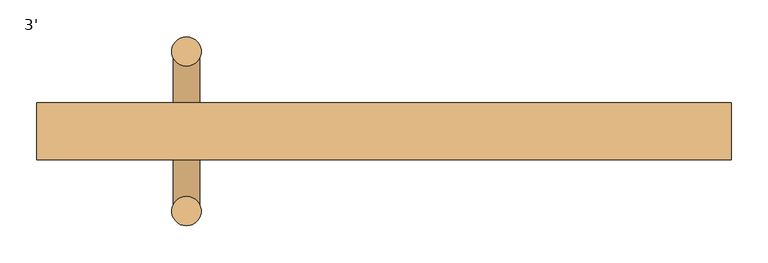
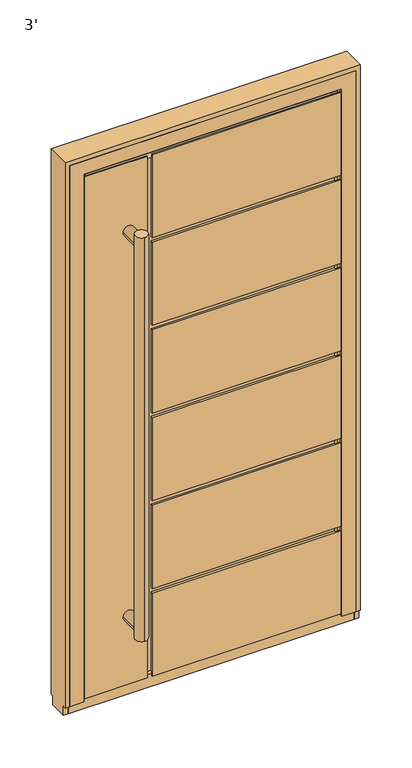
"""IFC4 building model written with IfcOpenShell, lengths in millimetres: door geometry, 3'."""

from ifc_helpers import new_model, si_unit, point, frame, frame_2d, origin, place, context, project, spatial, circle_curve, trimmed, segment, composite_curve, outline, extrude, faceted_brep, source, transform, mapped, element, save


def door_3_3562bf2b(model_context):
    return source(origin(), model_context, "Body", "SolidModel", [
        extrude(outline(composite_curve([segment(trimmed(circle_curve(frame_2d((-268.65, 52.7003001)), 20.0), [point((-268.65, 32.7003001))], [point((-268.65, 72.7003001))], False, "CARTESIAN"), True, "CONTINUOUS"), segment(trimmed(circle_curve(frame_2d((-268.65, 52.7003001)), 20.0), [point((-268.65, 72.7003001))], [point((-268.65, 32.7003001))], False, "CARTESIAN"), True, "CONTINUOUS")], self_intersect=False)), frame((0.0, 0.0, 210.0000003), z_axis=(0.0, 0.0, 1.0), x_axis=(1.0, 0.0, 0.0)), (0.0, 0.0, 1.0), 1363.8),
        extrude(outline(composite_curve([segment(trimmed(circle_curve(frame_2d((-268.65, -164.3003001)), 20.0), [point((-268.65, -184.3003001))], [point((-268.65, -144.3003001))], False, "CARTESIAN"), True, "CONTINUOUS"), segment(trimmed(circle_curve(frame_2d((-268.65, -164.3003001)), 20.0), [point((-268.65, -144.3003001))], [point((-268.65, -184.3003001))], False, "CARTESIAN"), True, "CONTINUOUS")], self_intersect=False)), frame((0.0, 0.0, 210.0000003), z_axis=(0.0, 0.0, 1.0), x_axis=(1.0, 0.0, 0.0)), (0.0, 0.0, 1.0), 1363.8),
        extrude(outline(composite_curve([segment(trimmed(circle_curve(frame_2d((241.9000003, -268.65)), 18.0), [point((241.9000003, -286.65))], [point((241.9000003, -250.65))], False, "CARTESIAN"), True, "CONTINUOUS"), segment(trimmed(circle_curve(frame_2d((241.9000003, -268.65)), 18.0), [point((241.9000003, -250.65))], [point((241.9000003, -286.65))], False, "CARTESIAN"), True, "CONTINUOUS")], self_intersect=False)), frame((0.0, -164.3, 0.0), z_axis=(0.0, 1.0, 0.0), x_axis=(0.0, 0.0, 1.0)), (0.0, 0.0, 1.0), 217.0),
        extrude(outline(composite_curve([segment(trimmed(circle_curve(frame_2d((1541.9000003, -268.65)), 18.0), [point((1541.9000003, -286.65))], [point((1541.9000003, -250.65))], False, "CARTESIAN"), True, "CONTINUOUS"), segment(trimmed(circle_curve(frame_2d((1541.9000003, -268.65)), 18.0), [point((1541.9000003, -250.65))], [point((1541.9000003, -286.65))], False, "CARTESIAN"), True, "CONTINUOUS")], self_intersect=False)), frame((0.0, -164.3, 0.0), z_axis=(0.0, 1.0, 0.0), x_axis=(0.0, 0.0, 1.0)), (0.0, 0.0, 1.0), 217.0),
        faceted_brep([(-193.65, -24.3, 306.466667), (383.65, -24.3, 306.466667), (383.65, -24.3, 291.466667), (-193.65, -24.3, 291.466667), (-193.65, -24.3, 35.0), (-208.65, -24.3, 35.0), (-208.65, -24.3, 1748.8000003), (-193.65, -24.3, 1748.8000003), (-193.65, -24.3, 1492.3333337), (383.65, -24.3, 1492.3333337), (383.65, -24.3, 1477.3333337), (-193.65, -24.3, 1477.3333337), (-193.65, -24.3, 1195.866667), (383.65, -24.3, 1195.866667), (383.65, -24.3, 1180.866667), (-193.65, -24.3, 1180.866667), (-193.65, -24.3, 899.4000004), (383.65, -24.3, 899.4000004), (383.65, -24.3, 884.4000004), (-193.65, -24.3, 884.4000004), (-193.65, -24.3, 602.9333337), (383.65, -24.3, 602.9333337), (383.65, -24.3, 587.9333337), (-193.65, -24.3, 587.9333337), (-193.65, -17.3, 587.9333337), (-193.65, -17.3, 306.466667), (383.65, -17.3, 587.9333337), (383.65, -26.3002302, 1748.8000003), (383.65, -26.3002302, 35.0), (383.65, -19.2979528, 35.0), (383.65, -19.2979528, 24.0), (383.65, -17.3, 24.0), (383.65, -17.3, 291.466667), (383.65, -17.3, 306.466667), (383.65, -17.3, 602.9333337), (383.65, -17.3, 884.4000004), (383.65, -17.3, 899.4000004), (383.65, -17.3, 1180.866667), (383.65, -17.3, 1195.866667), (383.65, -17.3, 1477.3333337), (383.65, -17.3, 1492.3333337), (383.65, -17.3, 1748.8000003), (-193.65, -17.3, 602.9333337), (-193.65, -17.3, 884.4000004), (-193.65, -17.3, 899.4000004), (-193.65, -17.3, 1180.866667), (-208.65, -19.2979528, 35.0), (-208.65, -19.2979528, 24.0), (-208.65, -17.3, 24.0), (-208.65, -17.3, 1748.8000003), (-383.65, -26.3002302, 35.0), (-383.65, -19.2979528, 35.0), (-193.65, -19.2979528, 35.0), (-193.65, -17.3, 291.466667), (-193.65, -17.3, 24.0), (-193.65, -19.2979528, 24.0), (-383.65, -19.2979528, 24.0), (-383.65, -17.3, 24.0), (-383.65, -17.3, 1748.8000003), (-193.65, -17.3, 1195.866667), (-193.65, -17.3, 1477.3333337), (-193.65, -17.3, 1492.3333337), (-193.65, -17.3, 1748.8000003), (408.65, -94.3, 10.0000003), (-193.65, -94.3, 10.0000003), (-193.65, -91.3, 10.0000003), (408.65, -91.3, 10.0000003), (-408.65, -91.3, 10.0000003), (-208.65, -91.3, 10.0000003), (-208.65, -94.3, 10.0000003), (-408.65, -94.3, 10.0000003), (408.65, -94.3, 306.466667), (408.65, -91.3, 306.466667), (408.65, -91.3, 587.9333337), (408.65, -94.3, 587.9333337), (408.65, -94.3, 899.4000004), (408.65, -91.3, 899.4000004), (408.65, -91.3, 1180.866667), (408.65, -94.3, 1180.866667), (408.65, -94.3, 602.9333337), (408.65, -91.3, 602.9333337), (408.65, -91.3, 884.4000004), (408.65, -94.3, 884.4000004), (408.65, -94.3, 1195.866667), (408.65, -91.3, 1195.866667), (408.65, -91.3, 1477.3333337), (408.65, -94.3, 1477.3333337), (408.65, -94.3, 1773.8000003), (408.65, -94.3, 1492.3333337), (408.65, -91.3, 1492.3333337), (408.65, -91.3, 1773.8000003), (408.65, -91.3, 291.466667), (408.65, -94.3, 291.466667), (-193.65, -91.3, 25.5), (393.15, -91.3, 25.5), (393.15, -91.3, 291.466667), (393.15, -91.3, 306.466667), (393.15, -91.3, 587.9333337), (393.15, -91.3, 899.4000004), (393.15, -91.3, 1180.866667), (393.15, -91.3, 602.9333337), (393.15, -91.3, 884.4000004), (-393.15, -91.3, 25.5), (-208.65, -91.3, 25.5), (-408.65, -91.3, 1773.8000003), (-208.65, -91.3, 1773.8000003), (-208.65, -91.3, 1758.3000003), (-393.15, -91.3, 1758.3000003), (393.15, -91.3, 1195.866667), (393.15, -91.3, 1477.3333337), (393.15, -91.3, 1492.3333337), (393.15, -91.3, 1758.3000003), (-193.65, -91.3, 1758.3000003), (-193.65, -91.3, 1773.8000003), (-193.65, -87.3, 291.466667), (-193.65, -87.3, 25.5), (-193.65, -94.3, 291.466667), (-208.65, -94.3, 1773.8000003), (-408.65, -94.3, 1773.8000003), (-193.65, -94.3, 587.9333337), (-193.65, -94.3, 306.466667), (-193.65, -94.3, 1180.866667), (-193.65, -94.3, 899.4000004), (-193.65, -94.3, 884.4000004), (-193.65, -94.3, 602.9333337), (-193.65, -94.3, 1477.3333337), (-193.65, -94.3, 1195.866667), (-193.65, -94.3, 1773.8000003), (-193.65, -94.3, 1492.3333337), (-208.65, -87.3, 1758.3000003), (-208.65, -87.3, 25.5), (-383.65, -26.3002302, 1748.8000003), (393.15, -26.3002302, 1758.3000003), (393.15, -26.3002302, 25.5), (-393.15, -26.3002302, 25.5), (-393.15, -26.3002302, 1758.3000003), (393.15, -87.3, 1492.3333337), (393.15, -87.3, 1477.3333337), (393.15, -87.3, 1195.866667), (393.15, -87.3, 1180.866667), (393.15, -87.3, 899.4000004), (393.15, -87.3, 884.4000004), (393.15, -87.3, 602.9333337), (393.15, -87.3, 587.9333337), (393.15, -87.3, 306.466667), (393.15, -87.3, 291.466667), (-193.65, -87.3, 1477.3333337), (-193.65, -87.3, 1492.3333337), (-193.65, -87.3, 1758.3000003), (-193.65, -87.3, 306.466667), (-193.65, -87.3, 587.9333337), (-193.65, -87.3, 602.9333337), (-193.65, -87.3, 884.4000004), (-193.65, -87.3, 899.4000004), (-193.65, -87.3, 1180.866667), (-193.65, -87.3, 1195.866667)], [[[0, 1, 2, 3, 4, 5, 6, 7, 8, 9, 10, 11, 12, 13, 14, 15, 16, 17, 18, 19, 20, 21, 22, 23]], [[23, 24, 25, 0]], [[23, 22, 26, 24]], [[27, 28, 29, 30, 31, 32, 2, 1, 33, 26, 22, 21, 34, 35, 18, 17, 36, 37, 14, 13, 38, 39, 10, 9, 40, 41]], [[42, 34, 21, 20]], [[19, 43, 42, 20]], [[19, 18, 35, 43]], [[44, 36, 17, 16]], [[15, 45, 44, 16]], [[5, 46, 47, 48, 49, 6]], [[28, 50, 51, 46, 5, 4, 52, 29]], [[53, 54, 55, 52, 4, 3]], [[3, 2, 32, 53]], [[25, 33, 1, 0]], [[29, 52, 55, 30]], [[56, 47, 46, 51]], [[30, 55, 54, 31]], [[57, 48, 47, 56]], [[36, 44, 45, 37]], [[34, 42, 43, 35]], [[33, 25, 24, 26]], [[54, 53, 32, 31]], [[58, 49, 48, 57]], [[38, 59, 60, 39]], [[41, 40, 61, 62]], [[63, 64, 65, 66]], [[67, 68, 69, 70]], [[71, 72, 73, 74]], [[75, 76, 77, 78]], [[79, 80, 81, 82]], [[83, 84, 85, 86]], [[87, 88, 89, 90]], [[66, 91, 92, 63]], [[65, 93, 94, 95, 91, 66]], [[72, 96, 97, 73]], [[76, 98, 99, 77]], [[80, 100, 101, 81]], [[102, 103, 68, 67, 104, 105, 106, 107]], [[84, 108, 109, 85]], [[90, 89, 110, 111, 112, 113]], [[114, 115, 93, 65, 64, 116]], [[70, 69, 117, 118]], [[63, 92, 116, 64]], [[74, 119, 120, 71]], [[78, 121, 122, 75]], [[82, 123, 124, 79]], [[86, 125, 126, 83]], [[87, 127, 128, 88]], [[70, 118, 104, 67]], [[129, 106, 105, 117, 69, 68, 103, 130]], [[58, 57, 56, 51, 50, 131]], [[132, 133, 134, 135], [131, 50, 28, 27]], [[111, 110, 136, 137, 109, 108, 138, 139, 99, 98, 140, 141, 101, 100, 142, 143, 97, 96, 144, 145, 95, 94, 133, 132]], [[94, 93, 115, 130, 103, 102, 134, 133]], [[135, 134, 102, 107]], [[146, 137, 136, 147, 148, 129, 130, 115, 114, 145, 144, 149, 150, 143, 142, 151, 152, 141, 140, 153, 154, 139, 138, 155]], [[153, 122, 121, 154]], [[153, 140, 98, 76, 75, 122]], [[123, 82, 81, 101, 141, 152]], [[151, 124, 123, 152]], [[151, 142, 100, 80, 79, 124]], [[119, 74, 73, 97, 143, 150]], [[149, 120, 119, 150]], [[149, 144, 96, 72, 71, 120]], [[116, 92, 91, 95, 145, 114]], [[15, 14, 37, 45]], [[59, 38, 13, 12]], [[11, 60, 59, 12]], [[11, 10, 39, 60]], [[61, 40, 9, 8]], [[8, 7, 62, 61]], [[125, 86, 85, 109, 137, 146]], [[128, 127, 113, 112, 148, 147]], [[121, 78, 77, 99, 139, 154]], [[155, 138, 108, 84, 83, 126]], [[155, 126, 125, 146]], [[147, 136, 110, 89, 88, 128]], [[90, 113, 127, 87]], [[118, 117, 105, 104]], [[132, 135, 107, 106, 129, 148, 112, 111]], [[27, 41, 62, 7, 6, 49, 58, 131]]]),
        faceted_brep([(-457.2, -94.3, 0.0), (-457.2, -85.2997571, 0.0), (-412.7, -85.2997571, 0.0), (-412.7, -94.3, 0.0), (-403.2, -21.8000042, 0.0), (-403.2, -26.3, 0.0), (-457.2, -26.3, 0.0), (-457.2, -17.3, 0.0), (-387.7, -17.3, 0.0), (-387.7, -21.8000042, 0.0), (457.2, -17.3, 0.0), (457.2, -26.3, 0.0), (403.2, -26.3, 0.0), (403.2, -21.8000042, 0.0), (387.7, -21.8000042, 0.0), (387.7, -17.3, 0.0), (412.7, -85.2997571, 0.0), (457.2, -85.2997571, 0.0), (457.2, -94.3, 0.0), (412.7, -94.3, 0.0), (-457.2, -26.3, -30.0), (-457.2, -85.2997571, -30.0), (-457.2, -94.3, 1828.8), (-457.2, -17.3, 1828.8), (-412.7, -94.3, 1784.3), (412.7, -94.3, 1784.3), (457.2, -94.3, 1828.8), (457.2, -17.3, 1828.8), (457.2, -85.2997571, -30.0), (457.2, -26.3, -30.0), (387.7, -17.3, 1759.3), (-387.7, -17.3, 1759.3), (-403.2, -85.3, 1774.8), (-403.2, -85.3, 14.5), (-403.2, -26.3, 14.5), (-403.2, -21.8000042, 1774.8), (403.2, -21.8000042, 1774.8), (403.2, -85.3, 1774.8), (403.2, -26.3, 14.5), (403.2, -85.3, 14.5), (-412.7, -85.3, 1784.3), (412.7, -85.3, 1784.3), (-387.7, -21.8000042, 1759.3), (387.7, -21.8000042, 1759.3)], [[[0, 1, 2, 3]], [[4, 5, 6, 7, 8, 9]], [[10, 11, 12, 13, 14, 15]], [[16, 17, 18, 19]], [[7, 6, 20, 21, 1, 0, 22, 23]], [[3, 24, 25, 19, 18, 26, 22, 0]], [[22, 26, 27, 23]], [[18, 17, 28, 29, 11, 10, 27, 26]], [[7, 23, 27, 10, 15, 30, 31, 8]], [[32, 33, 34, 5, 4, 35]], [[35, 36, 37, 32]], [[36, 13, 12, 38, 39, 37]], [[40, 24, 3, 2]], [[16, 41, 40, 2, 1, 21, 28, 17], [37, 39, 33, 32]], [[9, 42, 43, 14, 13, 36, 35, 4]], [[8, 31, 42, 9]], [[24, 40, 41, 25]], [[30, 43, 42, 31]], [[19, 25, 41, 16]], [[14, 43, 30, 15]], [[20, 6, 5, 34, 38, 12, 11, 29]], [[39, 38, 34, 33]], [[20, 29, 28, 21]]]),
        faceted_brep([(-457.2, -85.3, -30.0), (-472.2, -85.3, -30.0), (-472.2, -26.3, -30.0), (-457.2, -26.3, -30.0), (-457.2, -94.3, 1828.8), (-457.2, -94.3, 0.0), (-457.2, -85.3, 0.0), (-457.2, -26.3, 0.0), (-457.2, -17.3, 0.0), (-457.2, -17.3, 1828.8), (-472.2, -26.3, 0.0), (472.2, -26.3, 0.0), (472.2, -26.3, -30.0), (457.2, -26.3, -30.0), (457.2, -26.3, 0.0), (-472.2, -17.3, 1843.8), (-472.2, -17.3, 0.0), (-472.2, -85.3, 0.0), (-472.2, -94.3, 0.0), (-472.2, -94.3, 1843.8), (457.2, -85.3, 0.0), (457.2, -85.3, -30.0), (472.2, -85.3, -30.0), (472.2, -85.3, 0.0), (457.2, -17.3, 1828.8), (457.2, -17.3, 0.0), (457.2, -94.3, 0.0), (457.2, -94.3, 1828.8), (472.2, -94.3, 0.0), (472.2, -94.3, 1843.8), (472.2, -17.3, 0.0), (472.2, -17.3, 1843.8)], [[[0, 1, 2, 3]], [[4, 5, 6, 0, 3, 7, 8, 9]], [[7, 3, 2, 10]], [[11, 12, 13, 14]], [[15, 16, 10, 2, 1, 17, 18, 19]], [[17, 1, 0, 6]], [[20, 21, 22, 23]], [[24, 25, 14, 13, 21, 20, 26, 27]], [[27, 26, 28, 29, 19, 18, 5, 4]], [[6, 5, 18, 17]], [[23, 28, 26, 20]], [[22, 21, 13, 12]], [[10, 16, 8, 7]], [[14, 25, 30, 11]], [[9, 8, 16, 15, 31, 30, 25, 24]], [[29, 28, 23, 22, 12, 11, 30, 31]], [[9, 24, 27, 4]], [[19, 29, 31, 15]]]),
    ])


if __name__ == "__main__":
    model = new_model("IFC4")
    model_context = context("Model", 3, world=origin())
    ifc_project = project(units=[si_unit("LENGTHUNIT", "METRE", prefix="MILLI")], contexts=[model_context])
    site = spatial("IfcSite", under=ifc_project)
    building = spatial("IfcBuilding", under=site)
    placement = place(None, origin())
    door_3_shape = door_3_3562bf2b(model_context)
    element("IfcDoor", 1, ObjectType="3'", at=placement, inside=building, context=model_context, shape_type="MappedRepresentation", body=[
        mapped(door_3_shape, transform((0.0, 0.0, 0.0), x_axis=(1.0, 0.0, 0.0), y_axis=(0.0, 1.0, 0.0), z_axis=(0.0, 0.0, 1.0))),
    ])
    save(model, "model.ifc")

# Revit data of these elements
# Type "3'"
#   Type Mark = "41"
#   Water resistance = "up to Class E900, EN 12208:2001"
#   Uniclass2015Version = "v1.21"
#   Uniclass2015Reference = "Ss_25_30_20_30"
#   Uniclass2015Description = "Frame and door leaf system"
#   URL = "www.aluprof.com"
#   Type IFC Predefined Type = "USERDEFINED"
#   Right-hand / Left-hand door [instance default] = ""
#   Resistance to wind load = "up to Class C5/B5, EN 12210:2001"
#   Insert type = "ST"
#   Hardware [instance default] = ""
#   Product page = "https://aluprof.com/en/architects/offer/window-and-door-systems/panel-doors#visualisation"
#   Operation = "SinglePanelOutwardOpening"
#   Opening type = "Outward"
#   NBSReference = "25-50-20/125"
#   NBSDescription = "Frame and door leaf system"
#   Important = "The actual acceptable construction dimensions are dependent on the selection of profiles and hardware, glazing type, construction weight and the construction’s operating conditions. These should be determined by a suitably qualified person, and using ALUPROF’s calculation software"
#   IfcExportType = "USERDEFINED"
#   IfcExportAs = "IfcDoorType"
#   Handle type [instance default] = ""
#   Manufacturer = "ALUPROF SA"
#   Export Type to IFC As = "IfcDoorType"
#   Door sill type [instance default] = ""
#   Description = "External single-leaf panel door outward opening"
#   Model = "MB-86 ST Panel Door AD07"
#   Content of the recyclate in the material = "69.2%"
#   COBie.Type.WarrantyDurationParts = ""
#   COBie.Type.Name = ""
#   COBie.Type.Manufacturer = "ALUPROF SA"
#   COBie.Space.Name = ""
#   COBie.Floor.Name = ""
#   COBie.Facility.Name = ""
#   COBie.CreatedOn = ""
#   COBie.Component.WarrantyStartDate = ""
#   COBie.Component.Name = "MB-86 ST Panel Door AD07"
#   Burglar resistance = "RC2"
#   Air permeability = "up to Class 4, EN 12207:2001"
#   Width of the active leaf = 2' - 8.17717"
#   Placement in wall = 0' - 0.7874"
#   Thickness = 0' - 3.0315"
#   Height of the opening sash = 5' - 9.44094"
#   Handle Offset = 3' - 5.33858"
#   Rough Height = 6' - 2.40945"
#   Rough Width = 3' - 1.1811"
#   Height = 6' - 0"
#   Width = 3' - 0"
#   Construction depth = 0' - 3.0315"
#   Clear opening width = 2' - 3.94882"
#   Clear opening height = 5' - 8.47638"
#   Height of the array = 0' - 11.08136"
#   Schedule No. [instance default] = 1
#   Handrail [instance default] = yes
#   IsExternal = yes
#   Handle [instance default] = no
#   Door closer [instance default] = no
#   Function = 1
#   COBie.Type = yes
#   COBie = yes
#   Access control [instance default] = no
#   Panel = element 361060
#   Wall Closure = (empty or 0)
